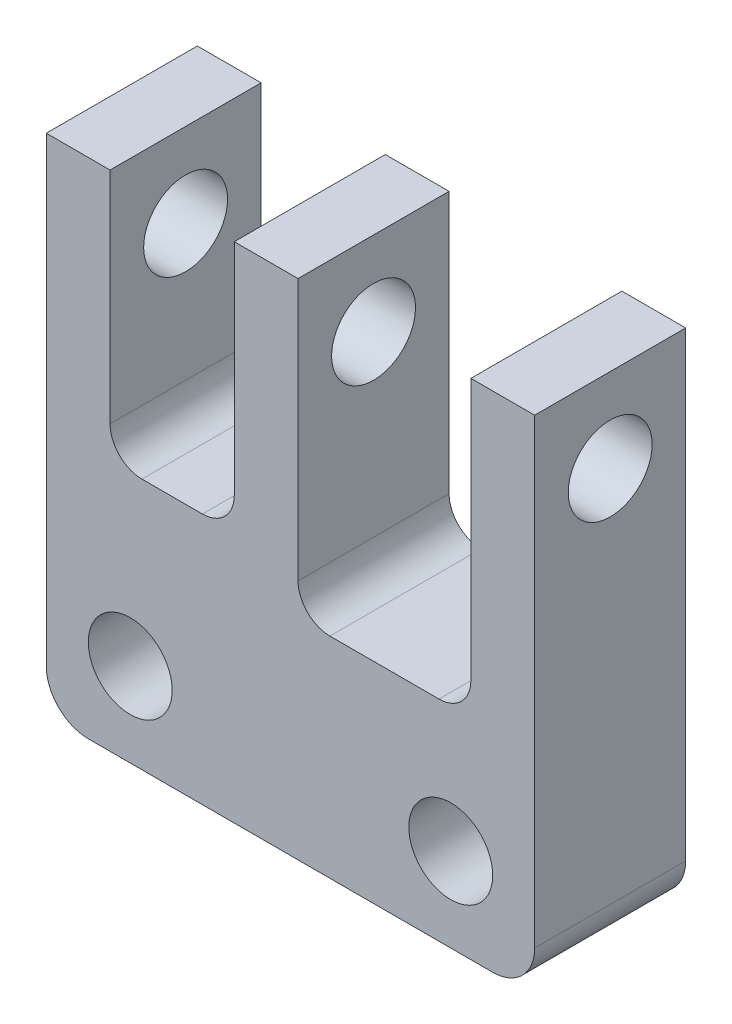
ISO-10303-21;
HEADER;
FILE_DESCRIPTION(('STEP AP214'),'2;1');
FILE_NAME('part.step','',(''),(''),'','','');
FILE_SCHEMA(('AUTOMOTIVE_DESIGN { 1 0 10303 214 1 1 1 1 }'));
ENDSEC;
DATA;
#1=APPLICATION_CONTEXT('core data for automotive mechanical design processes');
#2=APPLICATION_PROTOCOL_DEFINITION('international standard','automotive_design',2000,#1);
#3=PRODUCT_CONTEXT('',#1,'mechanical');
#4=PRODUCT('Part','Part','',(#3));
#5=PRODUCT_RELATED_PRODUCT_CATEGORY('part','',(#4));
#6=PRODUCT_DEFINITION_FORMATION('','',#4);
#7=PRODUCT_DEFINITION_CONTEXT('part definition',#1,'design');
#8=PRODUCT_DEFINITION('design','',#6,#7);
#9=PRODUCT_DEFINITION_SHAPE('','',#8);
#10=(LENGTH_UNIT() NAMED_UNIT(*) SI_UNIT(.MILLI.,.METRE.));
#11=(NAMED_UNIT(*) PLANE_ANGLE_UNIT() SI_UNIT($,.RADIAN.));
#12=(NAMED_UNIT(*) SI_UNIT($,.STERADIAN.) SOLID_ANGLE_UNIT());
#13=UNCERTAINTY_MEASURE_WITH_UNIT(LENGTH_MEASURE(1.E-05),#10,'distance_accuracy_value','');
#14=(GEOMETRIC_REPRESENTATION_CONTEXT(3) GLOBAL_UNCERTAINTY_ASSIGNED_CONTEXT((#13)) GLOBAL_UNIT_ASSIGNED_CONTEXT((#10,
#11,#12)) REPRESENTATION_CONTEXT('',''));
#15=CARTESIAN_POINT('',(0.,0.,0.));
#16=DIRECTION('',(0.,0.,1.));
#17=DIRECTION('',(1.,0.,0.));
#18=AXIS2_PLACEMENT_3D('',#15,#16,#17);
#19=CARTESIAN_POINT('',(0.,3.,0.));
#20=DIRECTION('',(0.,-1.,0.));
#21=DIRECTION('',(0.,0.,-1.));
#22=AXIS2_PLACEMENT_3D('',#19,#20,#21);
#23=PLANE('',#22);
#24=DIRECTION('',(-1.,0.,0.));
#25=VECTOR('',#24,1.);
#26=CARTESIAN_POINT('',(-1.455,3.,-0.45));
#27=LINE('',#26,#25);
#28=CARTESIAN_POINT('',(0.0450000000000003,3.,-0.45));
#29=VERTEX_POINT('',#28);
#30=CARTESIAN_POINT('',(-0.335,3.,-0.45));
#31=VERTEX_POINT('',#30);
#32=EDGE_CURVE('E209',#29,#31,#27,.T.);
#33=ORIENTED_EDGE('',*,*,#32,.T.);
#34=DIRECTION('',(0.,0.,1.));
#35=VECTOR('',#34,1.);
#36=CARTESIAN_POINT('',(-0.335,3.,0.));
#37=LINE('',#36,#35);
#38=CARTESIAN_POINT('',(-0.335,3.,0.45));
#39=VERTEX_POINT('',#38);
#40=EDGE_CURVE('E11',#31,#39,#37,.T.);
#41=ORIENTED_EDGE('',*,*,#40,.T.);
#42=DIRECTION('',(1.,0.,0.));
#43=VECTOR('',#42,1.);
#44=CARTESIAN_POINT('',(-1.455,3.,0.45));
#45=LINE('',#44,#43);
#46=CARTESIAN_POINT('',(0.0450000000000003,3.,0.45));
#47=VERTEX_POINT('',#46);
#48=EDGE_CURVE('E193',#39,#47,#45,.T.);
#49=ORIENTED_EDGE('',*,*,#48,.T.);
#50=DIRECTION('',(0.,0.,-1.));
#51=VECTOR('',#50,1.);
#52=CARTESIAN_POINT('',(0.0450000000000003,3.,0.));
#53=LINE('',#52,#51);
#54=EDGE_CURVE('E390',#47,#29,#53,.T.);
#55=ORIENTED_EDGE('',*,*,#54,.T.);
#56=EDGE_LOOP('',(#33,#41,#49,#55));
#57=FACE_BOUND('',#56,.T.);
#58=ADVANCED_FACE('F43',(#57),#23,.F.);
#59=CARTESIAN_POINT('',(1.455,3.,-0.45));
#60=VERTEX_POINT('',#59);
#61=CARTESIAN_POINT('',(1.075,3.,-0.45));
#62=VERTEX_POINT('',#61);
#63=EDGE_CURVE('E208',#60,#62,#27,.T.);
#64=ORIENTED_EDGE('',*,*,#63,.T.);
#65=DIRECTION('',(0.,0.,1.));
#66=VECTOR('',#65,1.);
#67=CARTESIAN_POINT('',(1.075,3.,0.));
#68=LINE('',#67,#66);
#69=CARTESIAN_POINT('',(1.075,3.,0.45));
#70=VERTEX_POINT('',#69);
#71=EDGE_CURVE('E179',#62,#70,#68,.T.);
#72=ORIENTED_EDGE('',*,*,#71,.T.);
#73=CARTESIAN_POINT('',(1.455,3.,0.45));
#74=VERTEX_POINT('',#73);
#75=EDGE_CURVE('E198',#70,#74,#45,.T.);
#76=ORIENTED_EDGE('',*,*,#75,.T.);
#77=DIRECTION('',(0.,0.,-1.));
#78=VECTOR('',#77,1.);
#79=CARTESIAN_POINT('',(1.455,3.,0.45));
#80=LINE('',#79,#78);
#81=EDGE_CURVE('E212',#74,#60,#80,.T.);
#82=ORIENTED_EDGE('',*,*,#81,.T.);
#83=EDGE_LOOP('',(#64,#72,#76,#82));
#84=FACE_BOUND('',#83,.T.);
#85=ADVANCED_FACE('F335',(#84),#23,.F.);
#86=CARTESIAN_POINT('',(1.455,3.,0.45));
#87=DIRECTION('',(-1.,0.,0.));
#88=DIRECTION('',(0.,0.,1.));
#89=AXIS2_PLACEMENT_3D('',#86,#87,#88);
#90=PLANE('',#89);
#91=CARTESIAN_POINT('',(1.455,2.5,0.));
#92=DIRECTION('',(1.,0.,0.));
#93=DIRECTION('',(0.,0.,-1.));
#94=AXIS2_PLACEMENT_3D('',#91,#92,#93);
#95=CIRCLE('',#94,0.25);
#96=CARTESIAN_POINT('',(1.455,2.5,-0.25));
#97=VERTEX_POINT('',#96);
#98=EDGE_CURVE('E305',#97,#97,#95,.T.);
#99=ORIENTED_EDGE('',*,*,#98,.F.);
#100=EDGE_LOOP('',(#99));
#101=FACE_BOUND('',#100,.T.);
#102=DIRECTION('',(0.,-1.,0.));
#103=VECTOR('',#102,1.);
#104=CARTESIAN_POINT('',(1.455,3.,0.45));
#105=LINE('',#104,#103);
#106=CARTESIAN_POINT('',(1.455,0.25,0.45));
#107=VERTEX_POINT('',#106);
#108=EDGE_CURVE('E195',#74,#107,#105,.T.);
#109=ORIENTED_EDGE('',*,*,#108,.T.);
#110=DIRECTION('',(0.,0.,-1.));
#111=VECTOR('',#110,1.);
#112=CARTESIAN_POINT('',(1.455,0.25,-0.45));
#113=LINE('',#112,#111);
#114=CARTESIAN_POINT('',(1.455,0.25,-0.45));
#115=VERTEX_POINT('',#114);
#116=EDGE_CURVE('E381',#107,#115,#113,.T.);
#117=ORIENTED_EDGE('',*,*,#116,.T.);
#118=DIRECTION('',(0.,-1.,0.));
#119=VECTOR('',#118,1.);
#120=CARTESIAN_POINT('',(1.455,3.,-0.45));
#121=LINE('',#120,#119);
#122=EDGE_CURVE('E397',#60,#115,#121,.T.);
#123=ORIENTED_EDGE('',*,*,#122,.F.);
#124=ORIENTED_EDGE('',*,*,#81,.F.);
#125=EDGE_LOOP('',(#109,#117,#123,#124));
#126=FACE_BOUND('',#125,.T.);
#127=ADVANCED_FACE('F338',(#101,#126),#90,.F.);
#128=CARTESIAN_POINT('',(-1.455,3.,-0.45));
#129=DIRECTION('',(0.,0.,1.));
#130=DIRECTION('',(1.,0.,0.));
#131=AXIS2_PLACEMENT_3D('',#128,#129,#130);
#132=PLANE('',#131);
#133=CARTESIAN_POINT('',(-0.955,0.5,-0.45));
#134=DIRECTION('',(0.,0.,1.));
#135=DIRECTION('',(1.,0.,0.));
#136=AXIS2_PLACEMENT_3D('',#133,#134,#135);
#137=CIRCLE('',#136,0.25);
#138=CARTESIAN_POINT('',(-0.705,0.5,-0.45));
#139=VERTEX_POINT('',#138);
#140=EDGE_CURVE('E266',#139,#139,#137,.T.);
#141=ORIENTED_EDGE('',*,*,#140,.T.);
#142=EDGE_LOOP('',(#141));
#143=FACE_BOUND('',#142,.T.);
#144=CARTESIAN_POINT('',(0.955,0.5,-0.45));
#145=DIRECTION('',(0.,0.,1.));
#146=DIRECTION('',(1.,0.,0.));
#147=AXIS2_PLACEMENT_3D('',#144,#145,#146);
#148=CIRCLE('',#147,0.25);
#149=CARTESIAN_POINT('',(1.205,0.5,-0.45));
#150=VERTEX_POINT('',#149);
#151=EDGE_CURVE('E285',#150,#150,#148,.T.);
#152=ORIENTED_EDGE('',*,*,#151,.T.);
#153=EDGE_LOOP('',(#152));
#154=FACE_BOUND('',#153,.T.);
#155=CARTESIAN_POINT('',(-0.525,1.69,-0.45));
#156=DIRECTION('',(0.,0.,1.));
#157=DIRECTION('',(1.,0.,0.));
#158=AXIS2_PLACEMENT_3D('',#155,#156,#157);
#159=CIRCLE('',#158,0.19);
#160=CARTESIAN_POINT('',(-0.525000000000001,1.5,-0.45));
#161=VERTEX_POINT('',#160);
#162=CARTESIAN_POINT('',(-0.335,1.69,-0.45));
#163=VERTEX_POINT('',#162);
#164=EDGE_CURVE('E220',#161,#163,#159,.T.);
#165=ORIENTED_EDGE('',*,*,#164,.T.);
#166=DIRECTION('',(0.,1.,0.));
#167=VECTOR('',#166,1.);
#168=CARTESIAN_POINT('',(-0.335,3.,-0.45));
#169=LINE('',#168,#167);
#170=EDGE_CURVE('E237',#163,#31,#169,.T.);
#171=ORIENTED_EDGE('',*,*,#170,.T.);
#172=ORIENTED_EDGE('',*,*,#32,.F.);
#173=DIRECTION('',(0.,-1.,0.));
#174=VECTOR('',#173,1.);
#175=CARTESIAN_POINT('',(0.0450000000000003,3.,-0.45));
#176=LINE('',#175,#174);
#177=CARTESIAN_POINT('',(0.0450000000000003,1.44,-0.45));
#178=VERTEX_POINT('',#177);
#179=EDGE_CURVE('E66',#29,#178,#176,.T.);
#180=ORIENTED_EDGE('',*,*,#179,.T.);
#181=CARTESIAN_POINT('',(0.235,1.44,-0.45));
#182=DIRECTION('',(0.,0.,1.));
#183=DIRECTION('',(1.,0.,0.));
#184=AXIS2_PLACEMENT_3D('',#181,#182,#183);
#185=CIRCLE('',#184,0.19);
#186=CARTESIAN_POINT('',(0.235000000000002,1.25,-0.45));
#187=VERTEX_POINT('',#186);
#188=EDGE_CURVE('E235',#178,#187,#185,.T.);
#189=ORIENTED_EDGE('',*,*,#188,.T.);
#190=DIRECTION('',(1.,0.,0.));
#191=VECTOR('',#190,1.);
#192=CARTESIAN_POINT('',(-1.455,1.25,-0.45));
#193=LINE('',#192,#191);
#194=CARTESIAN_POINT('',(0.884999999999999,1.25,-0.45));
#195=VERTEX_POINT('',#194);
#196=EDGE_CURVE('E230',#187,#195,#193,.T.);
#197=ORIENTED_EDGE('',*,*,#196,.T.);
#198=CARTESIAN_POINT('',(0.885,1.44,-0.45));
#199=DIRECTION('',(0.,0.,1.));
#200=DIRECTION('',(1.,0.,0.));
#201=AXIS2_PLACEMENT_3D('',#198,#199,#200);
#202=CIRCLE('',#201,0.19);
#203=CARTESIAN_POINT('',(1.075,1.44,-0.45));
#204=VERTEX_POINT('',#203);
#205=EDGE_CURVE('E227',#195,#204,#202,.T.);
#206=ORIENTED_EDGE('',*,*,#205,.T.);
#207=DIRECTION('',(0.,1.,0.));
#208=VECTOR('',#207,1.);
#209=CARTESIAN_POINT('',(1.075,3.,-0.45));
#210=LINE('',#209,#208);
#211=EDGE_CURVE('E238',#204,#62,#210,.T.);
#212=ORIENTED_EDGE('',*,*,#211,.T.);
#213=ORIENTED_EDGE('',*,*,#63,.F.);
#214=ORIENTED_EDGE('',*,*,#122,.T.);
#215=CARTESIAN_POINT('',(1.205,0.25,-0.45));
#216=DIRECTION('',(0.,0.,1.));
#217=DIRECTION('',(1.,0.,0.));
#218=AXIS2_PLACEMENT_3D('',#215,#216,#217);
#219=CIRCLE('',#218,0.25);
#220=CARTESIAN_POINT('',(1.205,0.,-0.45));
#221=VERTEX_POINT('',#220);
#222=EDGE_CURVE('E414',#115,#221,#219,.F.);
#223=ORIENTED_EDGE('',*,*,#222,.T.);
#224=DIRECTION('',(-1.,0.,0.));
#225=VECTOR('',#224,1.);
#226=CARTESIAN_POINT('',(-1.455,0.,-0.45));
#227=LINE('',#226,#225);
#228=CARTESIAN_POINT('',(-1.205,0.,-0.45));
#229=VERTEX_POINT('',#228);
#230=EDGE_CURVE('E219',#221,#229,#227,.T.);
#231=ORIENTED_EDGE('',*,*,#230,.T.);
#232=CARTESIAN_POINT('',(-1.205,0.25,-0.45));
#233=DIRECTION('',(0.,0.,1.));
#234=DIRECTION('',(1.,0.,0.));
#235=AXIS2_PLACEMENT_3D('',#232,#233,#234);
#236=CIRCLE('',#235,0.25);
#237=CARTESIAN_POINT('',(-1.455,0.25,-0.45));
#238=VERTEX_POINT('',#237);
#239=EDGE_CURVE('E404',#229,#238,#236,.F.);
#240=ORIENTED_EDGE('',*,*,#239,.T.);
#241=DIRECTION('',(0.,-1.,0.));
#242=VECTOR('',#241,1.);
#243=CARTESIAN_POINT('',(-1.455,3.,-0.45));
#244=LINE('',#243,#242);
#245=CARTESIAN_POINT('',(-1.455,3.,-0.45));
#246=VERTEX_POINT('',#245);
#247=EDGE_CURVE('E405',#246,#238,#244,.T.);
#248=ORIENTED_EDGE('',*,*,#247,.F.);
#249=CARTESIAN_POINT('',(-1.075,3.,-0.45));
#250=VERTEX_POINT('',#249);
#251=EDGE_CURVE('E215',#250,#246,#27,.T.);
#252=ORIENTED_EDGE('',*,*,#251,.F.);
#253=DIRECTION('',(0.,-1.,0.));
#254=VECTOR('',#253,1.);
#255=CARTESIAN_POINT('',(-1.075,3.,-0.45));
#256=LINE('',#255,#254);
#257=CARTESIAN_POINT('',(-1.075,1.69,-0.45));
#258=VERTEX_POINT('',#257);
#259=EDGE_CURVE('E56',#250,#258,#256,.T.);
#260=ORIENTED_EDGE('',*,*,#259,.T.);
#261=CARTESIAN_POINT('',(-0.885,1.69,-0.45));
#262=DIRECTION('',(0.,0.,1.));
#263=DIRECTION('',(1.,0.,0.));
#264=AXIS2_PLACEMENT_3D('',#261,#262,#263);
#265=CIRCLE('',#264,0.19);
#266=CARTESIAN_POINT('',(-0.884999999999999,1.5,-0.45));
#267=VERTEX_POINT('',#266);
#268=EDGE_CURVE('E221',#258,#267,#265,.T.);
#269=ORIENTED_EDGE('',*,*,#268,.T.);
#270=DIRECTION('',(1.,0.,0.));
#271=VECTOR('',#270,1.);
#272=CARTESIAN_POINT('',(-1.455,1.5,-0.45));
#273=LINE('',#272,#271);
#274=EDGE_CURVE('E222',#267,#161,#273,.T.);
#275=ORIENTED_EDGE('',*,*,#274,.T.);
#276=EDGE_LOOP('',(#165,#171,#172,#180,#189,#197,#206,#212,#213,#214,#223,#231,#240,#248,#252,
#260,#269,#275));
#277=FACE_BOUND('',#276,.T.);
#278=ADVANCED_FACE('F357',(#143,#154,#277),#132,.F.);
#279=CARTESIAN_POINT('',(-1.455,3.,0.45));
#280=DIRECTION('',(1.,0.,0.));
#281=DIRECTION('',(0.,0.,-1.));
#282=AXIS2_PLACEMENT_3D('',#279,#280,#281);
#283=PLANE('',#282);
#284=CARTESIAN_POINT('',(-1.455,2.5,0.));
#285=DIRECTION('',(1.,0.,0.));
#286=DIRECTION('',(0.,0.,-1.));
#287=AXIS2_PLACEMENT_3D('',#284,#285,#286);
#288=CIRCLE('',#287,0.25);
#289=CARTESIAN_POINT('',(-1.455,2.5,-0.25));
#290=VERTEX_POINT('',#289);
#291=EDGE_CURVE('E308',#290,#290,#288,.T.);
#292=ORIENTED_EDGE('',*,*,#291,.T.);
#293=EDGE_LOOP('',(#292));
#294=FACE_BOUND('',#293,.T.);
#295=ORIENTED_EDGE('',*,*,#247,.T.);
#296=DIRECTION('',(0.,0.,1.));
#297=VECTOR('',#296,1.);
#298=CARTESIAN_POINT('',(-1.455,0.25,0.45));
#299=LINE('',#298,#297);
#300=CARTESIAN_POINT('',(-1.455,0.25,0.45));
#301=VERTEX_POINT('',#300);
#302=EDGE_CURVE('E382',#238,#301,#299,.T.);
#303=ORIENTED_EDGE('',*,*,#302,.T.);
#304=DIRECTION('',(0.,-1.,0.));
#305=VECTOR('',#304,1.);
#306=CARTESIAN_POINT('',(-1.455,3.,0.45));
#307=LINE('',#306,#305);
#308=CARTESIAN_POINT('',(-1.455,3.,0.45));
#309=VERTEX_POINT('',#308);
#310=EDGE_CURVE('E196',#309,#301,#307,.T.);
#311=ORIENTED_EDGE('',*,*,#310,.F.);
#312=DIRECTION('',(0.,0.,1.));
#313=VECTOR('',#312,1.);
#314=CARTESIAN_POINT('',(-1.455,3.,0.45));
#315=LINE('',#314,#313);
#316=EDGE_CURVE('E194',#246,#309,#315,.T.);
#317=ORIENTED_EDGE('',*,*,#316,.F.);
#318=EDGE_LOOP('',(#295,#303,#311,#317));
#319=FACE_BOUND('',#318,.T.);
#320=ADVANCED_FACE('F352',(#294,#319),#283,.F.);
#321=CARTESIAN_POINT('',(-1.455,3.,0.45));
#322=DIRECTION('',(0.,0.,-1.));
#323=DIRECTION('',(-1.,0.,0.));
#324=AXIS2_PLACEMENT_3D('',#321,#322,#323);
#325=PLANE('',#324);
#326=CARTESIAN_POINT('',(-0.955,0.5,0.45));
#327=DIRECTION('',(0.,0.,1.));
#328=DIRECTION('',(1.,0.,0.));
#329=AXIS2_PLACEMENT_3D('',#326,#327,#328);
#330=CIRCLE('',#329,0.25);
#331=CARTESIAN_POINT('',(-0.705,0.5,0.45));
#332=VERTEX_POINT('',#331);
#333=EDGE_CURVE('E290',#332,#332,#330,.T.);
#334=ORIENTED_EDGE('',*,*,#333,.F.);
#335=EDGE_LOOP('',(#334));
#336=FACE_BOUND('',#335,.T.);
#337=CARTESIAN_POINT('',(0.955,0.5,0.45));
#338=DIRECTION('',(0.,0.,1.));
#339=DIRECTION('',(1.,0.,0.));
#340=AXIS2_PLACEMENT_3D('',#337,#338,#339);
#341=CIRCLE('',#340,0.25);
#342=CARTESIAN_POINT('',(1.205,0.5,0.45));
#343=VERTEX_POINT('',#342);
#344=EDGE_CURVE('E288',#343,#343,#341,.T.);
#345=ORIENTED_EDGE('',*,*,#344,.F.);
#346=EDGE_LOOP('',(#345));
#347=FACE_BOUND('',#346,.T.);
#348=ORIENTED_EDGE('',*,*,#48,.F.);
#349=DIRECTION('',(0.,1.,0.));
#350=VECTOR('',#349,1.);
#351=CARTESIAN_POINT('',(-0.335,1.69,0.45));
#352=LINE('',#351,#350);
#353=CARTESIAN_POINT('',(-0.335,1.69,0.45));
#354=VERTEX_POINT('',#353);
#355=EDGE_CURVE('E269',#354,#39,#352,.T.);
#356=ORIENTED_EDGE('',*,*,#355,.F.);
#357=CARTESIAN_POINT('',(-0.525,1.69,0.45));
#358=DIRECTION('',(0.,0.,1.));
#359=DIRECTION('',(1.,0.,0.));
#360=AXIS2_PLACEMENT_3D('',#357,#358,#359);
#361=CIRCLE('',#360,0.19);
#362=CARTESIAN_POINT('',(-0.525000000000001,1.5,0.45));
#363=VERTEX_POINT('',#362);
#364=EDGE_CURVE('E277',#363,#354,#361,.T.);
#365=ORIENTED_EDGE('',*,*,#364,.F.);
#366=DIRECTION('',(1.,0.,0.));
#367=VECTOR('',#366,1.);
#368=CARTESIAN_POINT('',(-0.884999999999999,1.5,0.45));
#369=LINE('',#368,#367);
#370=CARTESIAN_POINT('',(-0.884999999999999,1.5,0.45));
#371=VERTEX_POINT('',#370);
#372=EDGE_CURVE('E276',#371,#363,#369,.T.);
#373=ORIENTED_EDGE('',*,*,#372,.F.);
#374=CARTESIAN_POINT('',(-0.885,1.69,0.45));
#375=DIRECTION('',(0.,0.,1.));
#376=DIRECTION('',(1.,0.,0.));
#377=AXIS2_PLACEMENT_3D('',#374,#375,#376);
#378=CIRCLE('',#377,0.19);
#379=CARTESIAN_POINT('',(-1.075,1.69,0.45));
#380=VERTEX_POINT('',#379);
#381=EDGE_CURVE('E186',#380,#371,#378,.T.);
#382=ORIENTED_EDGE('',*,*,#381,.F.);
#383=DIRECTION('',(0.,-1.,0.));
#384=VECTOR('',#383,1.);
#385=CARTESIAN_POINT('',(-1.075,3.,0.45));
#386=LINE('',#385,#384);
#387=CARTESIAN_POINT('',(-1.075,3.,0.45));
#388=VERTEX_POINT('',#387);
#389=EDGE_CURVE('E171',#388,#380,#386,.T.);
#390=ORIENTED_EDGE('',*,*,#389,.F.);
#391=EDGE_CURVE('E181',#309,#388,#45,.T.);
#392=ORIENTED_EDGE('',*,*,#391,.F.);
#393=ORIENTED_EDGE('',*,*,#310,.T.);
#394=CARTESIAN_POINT('',(-1.205,0.25,0.45));
#395=DIRECTION('',(0.,0.,-1.));
#396=DIRECTION('',(-1.,0.,0.));
#397=AXIS2_PLACEMENT_3D('',#394,#395,#396);
#398=CIRCLE('',#397,0.25);
#399=CARTESIAN_POINT('',(-1.205,0.,0.45));
#400=VERTEX_POINT('',#399);
#401=EDGE_CURVE('E383',#301,#400,#398,.F.);
#402=ORIENTED_EDGE('',*,*,#401,.T.);
#403=DIRECTION('',(1.,0.,0.));
#404=VECTOR('',#403,1.);
#405=CARTESIAN_POINT('',(-1.455,0.,0.45));
#406=LINE('',#405,#404);
#407=CARTESIAN_POINT('',(1.205,0.,0.45));
#408=VERTEX_POINT('',#407);
#409=EDGE_CURVE('E216',#400,#408,#406,.T.);
#410=ORIENTED_EDGE('',*,*,#409,.T.);
#411=CARTESIAN_POINT('',(1.205,0.25,0.45));
#412=DIRECTION('',(0.,0.,-1.));
#413=DIRECTION('',(-1.,0.,0.));
#414=AXIS2_PLACEMENT_3D('',#411,#412,#413);
#415=CIRCLE('',#414,0.25);
#416=EDGE_CURVE('E378',#408,#107,#415,.F.);
#417=ORIENTED_EDGE('',*,*,#416,.T.);
#418=ORIENTED_EDGE('',*,*,#108,.F.);
#419=ORIENTED_EDGE('',*,*,#75,.F.);
#420=DIRECTION('',(0.,1.,0.));
#421=VECTOR('',#420,1.);
#422=CARTESIAN_POINT('',(1.075,3.,0.45));
#423=LINE('',#422,#421);
#424=CARTESIAN_POINT('',(1.075,1.44,0.45));
#425=VERTEX_POINT('',#424);
#426=EDGE_CURVE('E250',#425,#70,#423,.T.);
#427=ORIENTED_EDGE('',*,*,#426,.F.);
#428=CARTESIAN_POINT('',(0.885,1.44,0.45));
#429=DIRECTION('',(0.,0.,1.));
#430=DIRECTION('',(-1.,0.,0.));
#431=AXIS2_PLACEMENT_3D('',#428,#429,#430);
#432=CIRCLE('',#431,0.19);
#433=CARTESIAN_POINT('',(0.884999999999999,1.25,0.45));
#434=VERTEX_POINT('',#433);
#435=EDGE_CURVE('E255',#434,#425,#432,.T.);
#436=ORIENTED_EDGE('',*,*,#435,.F.);
#437=DIRECTION('',(1.,0.,0.));
#438=VECTOR('',#437,1.);
#439=CARTESIAN_POINT('',(0.884999999999999,1.25,0.45));
#440=LINE('',#439,#438);
#441=CARTESIAN_POINT('',(0.235000000000002,1.25,0.45));
#442=VERTEX_POINT('',#441);
#443=EDGE_CURVE('E260',#442,#434,#440,.T.);
#444=ORIENTED_EDGE('',*,*,#443,.F.);
#445=CARTESIAN_POINT('',(0.235,1.44,0.45));
#446=DIRECTION('',(0.,0.,1.));
#447=DIRECTION('',(-1.,0.,0.));
#448=AXIS2_PLACEMENT_3D('',#445,#446,#447);
#449=CIRCLE('',#448,0.19);
#450=CARTESIAN_POINT('',(0.0450000000000003,1.44,0.45));
#451=VERTEX_POINT('',#450);
#452=EDGE_CURVE('E257',#451,#442,#449,.T.);
#453=ORIENTED_EDGE('',*,*,#452,.F.);
#454=DIRECTION('',(0.,-1.,0.));
#455=VECTOR('',#454,1.);
#456=CARTESIAN_POINT('',(0.0450000000000003,1.44,0.45));
#457=LINE('',#456,#455);
#458=EDGE_CURVE('E263',#47,#451,#457,.T.);
#459=ORIENTED_EDGE('',*,*,#458,.F.);
#460=EDGE_LOOP('',(#348,#356,#365,#373,#382,#390,#392,#393,#402,#410,#417,#418,#419,#427,#436,
#444,#453,#459));
#461=FACE_BOUND('',#460,.T.);
#462=ADVANCED_FACE('F182',(#336,#347,#461),#325,.F.);
#463=ORIENTED_EDGE('',*,*,#391,.T.);
#464=DIRECTION('',(0.,0.,-1.));
#465=VECTOR('',#464,1.);
#466=CARTESIAN_POINT('',(-1.075,3.,0.));
#467=LINE('',#466,#465);
#468=EDGE_CURVE('E55',#388,#250,#467,.T.);
#469=ORIENTED_EDGE('',*,*,#468,.T.);
#470=ORIENTED_EDGE('',*,*,#251,.T.);
#471=ORIENTED_EDGE('',*,*,#316,.T.);
#472=EDGE_LOOP('',(#463,#469,#470,#471));
#473=FACE_BOUND('',#472,.T.);
#474=ADVANCED_FACE('F188',(#473),#23,.F.);
#475=CARTESIAN_POINT('',(0.,0.,0.));
#476=DIRECTION('',(0.,-1.,0.));
#477=DIRECTION('',(0.,0.,-1.));
#478=AXIS2_PLACEMENT_3D('',#475,#476,#477);
#479=PLANE('',#478);
#480=ORIENTED_EDGE('',*,*,#230,.F.);
#481=DIRECTION('',(0.,0.,-1.));
#482=VECTOR('',#481,1.);
#483=CARTESIAN_POINT('',(1.205,0.,0.45));
#484=LINE('',#483,#482);
#485=EDGE_CURVE('E377',#221,#408,#484,.F.);
#486=ORIENTED_EDGE('',*,*,#485,.T.);
#487=ORIENTED_EDGE('',*,*,#409,.F.);
#488=DIRECTION('',(0.,0.,1.));
#489=VECTOR('',#488,1.);
#490=CARTESIAN_POINT('',(-1.205,0.,-0.45));
#491=LINE('',#490,#489);
#492=EDGE_CURVE('E415',#400,#229,#491,.F.);
#493=ORIENTED_EDGE('',*,*,#492,.T.);
#494=EDGE_LOOP('',(#480,#486,#487,#493));
#495=FACE_BOUND('',#494,.T.);
#496=ADVANCED_FACE('F343',(#495),#479,.T.);
#497=CARTESIAN_POINT('',(1.205,0.25,0.45));
#498=DIRECTION('',(0.,0.,1.));
#499=DIRECTION('',(1.,0.,0.));
#500=AXIS2_PLACEMENT_3D('',#497,#498,#499);
#501=CYLINDRICAL_SURFACE('',#500,0.25);
#502=ORIENTED_EDGE('',*,*,#416,.F.);
#503=ORIENTED_EDGE('',*,*,#485,.F.);
#504=ORIENTED_EDGE('',*,*,#222,.F.);
#505=ORIENTED_EDGE('',*,*,#116,.F.);
#506=EDGE_LOOP('',(#502,#503,#504,#505));
#507=FACE_BOUND('',#506,.T.);
#508=ADVANCED_FACE('F349',(#507),#501,.T.);
#509=CARTESIAN_POINT('',(-1.205,0.25,0.45));
#510=DIRECTION('',(0.,0.,-1.));
#511=DIRECTION('',(-1.,0.,0.));
#512=AXIS2_PLACEMENT_3D('',#509,#510,#511);
#513=CYLINDRICAL_SURFACE('',#512,0.25);
#514=ORIENTED_EDGE('',*,*,#239,.F.);
#515=ORIENTED_EDGE('',*,*,#492,.F.);
#516=ORIENTED_EDGE('',*,*,#401,.F.);
#517=ORIENTED_EDGE('',*,*,#302,.F.);
#518=EDGE_LOOP('',(#514,#515,#516,#517));
#519=FACE_BOUND('',#518,.T.);
#520=ADVANCED_FACE('F44',(#519),#513,.T.);
#521=CARTESIAN_POINT('',(0.885,1.44,-2.55));
#522=DIRECTION('',(0.,0.,1.));
#523=DIRECTION('',(1.,0.,0.));
#524=AXIS2_PLACEMENT_3D('',#521,#522,#523);
#525=CYLINDRICAL_SURFACE('',#524,0.19);
#526=DIRECTION('',(0.,0.,1.));
#527=VECTOR('',#526,1.);
#528=CARTESIAN_POINT('',(0.884999999999999,1.25,-2.55));
#529=LINE('',#528,#527);
#530=EDGE_CURVE('E247',#195,#434,#529,.T.);
#531=ORIENTED_EDGE('',*,*,#530,.T.);
#532=ORIENTED_EDGE('',*,*,#435,.T.);
#533=DIRECTION('',(0.,0.,1.));
#534=VECTOR('',#533,1.);
#535=CARTESIAN_POINT('',(1.075,1.44,-2.55));
#536=LINE('',#535,#534);
#537=EDGE_CURVE('E187',#204,#425,#536,.T.);
#538=ORIENTED_EDGE('',*,*,#537,.F.);
#539=ORIENTED_EDGE('',*,*,#205,.F.);
#540=EDGE_LOOP('',(#531,#532,#538,#539));
#541=FACE_BOUND('',#540,.T.);
#542=ADVANCED_FACE('F373',(#541),#525,.F.);
#543=CARTESIAN_POINT('',(0.884999999999999,1.25,-2.55));
#544=DIRECTION('',(0.,-1.,0.));
#545=DIRECTION('',(1.,0.,0.));
#546=AXIS2_PLACEMENT_3D('',#543,#544,#545);
#547=PLANE('',#546);
#548=DIRECTION('',(0.,0.,1.));
#549=VECTOR('',#548,1.);
#550=CARTESIAN_POINT('',(0.235000000000002,1.25,-2.55));
#551=LINE('',#550,#549);
#552=EDGE_CURVE('E246',#187,#442,#551,.T.);
#553=ORIENTED_EDGE('',*,*,#552,.T.);
#554=ORIENTED_EDGE('',*,*,#443,.T.);
#555=ORIENTED_EDGE('',*,*,#530,.F.);
#556=ORIENTED_EDGE('',*,*,#196,.F.);
#557=EDGE_LOOP('',(#553,#554,#555,#556));
#558=FACE_BOUND('',#557,.T.);
#559=ADVANCED_FACE('F442',(#558),#547,.F.);
#560=CARTESIAN_POINT('',(0.235,1.44,-2.55));
#561=DIRECTION('',(0.,0.,1.));
#562=DIRECTION('',(1.,0.,0.));
#563=AXIS2_PLACEMENT_3D('',#560,#561,#562);
#564=CYLINDRICAL_SURFACE('',#563,0.19);
#565=DIRECTION('',(0.,0.,1.));
#566=VECTOR('',#565,1.);
#567=CARTESIAN_POINT('',(0.0450000000000003,1.44,-2.55));
#568=LINE('',#567,#566);
#569=EDGE_CURVE('E245',#178,#451,#568,.T.);
#570=ORIENTED_EDGE('',*,*,#569,.T.);
#571=ORIENTED_EDGE('',*,*,#452,.T.);
#572=ORIENTED_EDGE('',*,*,#552,.F.);
#573=ORIENTED_EDGE('',*,*,#188,.F.);
#574=EDGE_LOOP('',(#570,#571,#572,#573));
#575=FACE_BOUND('',#574,.T.);
#576=ADVANCED_FACE('F440',(#575),#564,.F.);
#577=CARTESIAN_POINT('',(1.075,3.,-2.55));
#578=DIRECTION('',(1.,0.,0.));
#579=DIRECTION('',(0.,1.,0.));
#580=AXIS2_PLACEMENT_3D('',#577,#578,#579);
#581=PLANE('',#580);
#582=CARTESIAN_POINT('',(1.075,2.5,0.));
#583=DIRECTION('',(1.,0.,0.));
#584=DIRECTION('',(0.,1.,0.));
#585=AXIS2_PLACEMENT_3D('',#582,#583,#584);
#586=CIRCLE('',#585,0.25);
#587=CARTESIAN_POINT('',(1.075,2.75,0.));
#588=VERTEX_POINT('',#587);
#589=EDGE_CURVE('E295',#588,#588,#586,.T.);
#590=ORIENTED_EDGE('',*,*,#589,.T.);
#591=EDGE_LOOP('',(#590));
#592=FACE_BOUND('',#591,.T.);
#593=ORIENTED_EDGE('',*,*,#537,.T.);
#594=ORIENTED_EDGE('',*,*,#426,.T.);
#595=ORIENTED_EDGE('',*,*,#71,.F.);
#596=ORIENTED_EDGE('',*,*,#211,.F.);
#597=EDGE_LOOP('',(#593,#594,#595,#596));
#598=FACE_BOUND('',#597,.T.);
#599=ADVANCED_FACE('F441',(#592,#598),#581,.F.);
#600=CARTESIAN_POINT('',(0.0450000000000003,1.44,-2.55));
#601=DIRECTION('',(-1.,0.,0.));
#602=DIRECTION('',(0.,0.,1.));
#603=AXIS2_PLACEMENT_3D('',#600,#601,#602);
#604=PLANE('',#603);
#605=CARTESIAN_POINT('',(0.0450000000000003,2.5,0.));
#606=DIRECTION('',(-1.,0.,0.));
#607=DIRECTION('',(0.,0.,1.));
#608=AXIS2_PLACEMENT_3D('',#605,#606,#607);
#609=CIRCLE('',#608,0.25);
#610=CARTESIAN_POINT('',(0.0450000000000003,2.5,0.25));
#611=VERTEX_POINT('',#610);
#612=EDGE_CURVE('E297',#611,#611,#609,.T.);
#613=ORIENTED_EDGE('',*,*,#612,.T.);
#614=EDGE_LOOP('',(#613));
#615=FACE_BOUND('',#614,.T.);
#616=ORIENTED_EDGE('',*,*,#54,.F.);
#617=ORIENTED_EDGE('',*,*,#458,.T.);
#618=ORIENTED_EDGE('',*,*,#569,.F.);
#619=ORIENTED_EDGE('',*,*,#179,.F.);
#620=EDGE_LOOP('',(#616,#617,#618,#619));
#621=FACE_BOUND('',#620,.T.);
#622=ADVANCED_FACE('F434',(#615,#621),#604,.F.);
#623=CARTESIAN_POINT('',(-0.525,1.69,-2.55));
#624=DIRECTION('',(0.,0.,1.));
#625=DIRECTION('',(1.,0.,0.));
#626=AXIS2_PLACEMENT_3D('',#623,#624,#625);
#627=CYLINDRICAL_SURFACE('',#626,0.19);
#628=DIRECTION('',(0.,0.,1.));
#629=VECTOR('',#628,1.);
#630=CARTESIAN_POINT('',(-0.525000000000001,1.5,-2.55));
#631=LINE('',#630,#629);
#632=EDGE_CURVE('E275',#161,#363,#631,.T.);
#633=ORIENTED_EDGE('',*,*,#632,.T.);
#634=ORIENTED_EDGE('',*,*,#364,.T.);
#635=DIRECTION('',(0.,0.,1.));
#636=VECTOR('',#635,1.);
#637=CARTESIAN_POINT('',(-0.335,1.69,-2.55));
#638=LINE('',#637,#636);
#639=EDGE_CURVE('E243',#163,#354,#638,.T.);
#640=ORIENTED_EDGE('',*,*,#639,.F.);
#641=ORIENTED_EDGE('',*,*,#164,.F.);
#642=EDGE_LOOP('',(#633,#634,#640,#641));
#643=FACE_BOUND('',#642,.T.);
#644=ADVANCED_FACE('F428',(#643),#627,.F.);
#645=CARTESIAN_POINT('',(-0.884999999999999,1.5,-2.55));
#646=DIRECTION('',(0.,-1.,0.));
#647=DIRECTION('',(0.,0.,-1.));
#648=AXIS2_PLACEMENT_3D('',#645,#646,#647);
#649=PLANE('',#648);
#650=DIRECTION('',(0.,0.,1.));
#651=VECTOR('',#650,1.);
#652=CARTESIAN_POINT('',(-0.884999999999999,1.5,-2.55));
#653=LINE('',#652,#651);
#654=EDGE_CURVE('E267',#267,#371,#653,.T.);
#655=ORIENTED_EDGE('',*,*,#654,.T.);
#656=ORIENTED_EDGE('',*,*,#372,.T.);
#657=ORIENTED_EDGE('',*,*,#632,.F.);
#658=ORIENTED_EDGE('',*,*,#274,.F.);
#659=EDGE_LOOP('',(#655,#656,#657,#658));
#660=FACE_BOUND('',#659,.T.);
#661=ADVANCED_FACE('F474',(#660),#649,.F.);
#662=CARTESIAN_POINT('',(-0.885,1.69,-2.55));
#663=DIRECTION('',(0.,0.,1.));
#664=DIRECTION('',(1.,0.,0.));
#665=AXIS2_PLACEMENT_3D('',#662,#663,#664);
#666=CYLINDRICAL_SURFACE('',#665,0.19);
#667=DIRECTION('',(0.,0.,1.));
#668=VECTOR('',#667,1.);
#669=CARTESIAN_POINT('',(-1.075,1.69,-2.55));
#670=LINE('',#669,#668);
#671=EDGE_CURVE('E270',#258,#380,#670,.T.);
#672=ORIENTED_EDGE('',*,*,#671,.T.);
#673=ORIENTED_EDGE('',*,*,#381,.T.);
#674=ORIENTED_EDGE('',*,*,#654,.F.);
#675=ORIENTED_EDGE('',*,*,#268,.F.);
#676=EDGE_LOOP('',(#672,#673,#674,#675));
#677=FACE_BOUND('',#676,.T.);
#678=ADVANCED_FACE('F482',(#677),#666,.F.);
#679=CARTESIAN_POINT('',(-0.335,1.69,-2.55));
#680=DIRECTION('',(1.,0.,0.));
#681=DIRECTION('',(0.,1.,0.));
#682=AXIS2_PLACEMENT_3D('',#679,#680,#681);
#683=PLANE('',#682);
#684=CARTESIAN_POINT('',(-0.335,2.5,0.));
#685=DIRECTION('',(1.,0.,0.));
#686=DIRECTION('',(0.,1.,0.));
#687=AXIS2_PLACEMENT_3D('',#684,#685,#686);
#688=CIRCLE('',#687,0.25);
#689=CARTESIAN_POINT('',(-0.335,2.75,0.));
#690=VERTEX_POINT('',#689);
#691=EDGE_CURVE('E300',#690,#690,#688,.T.);
#692=ORIENTED_EDGE('',*,*,#691,.T.);
#693=EDGE_LOOP('',(#692));
#694=FACE_BOUND('',#693,.T.);
#695=ORIENTED_EDGE('',*,*,#639,.T.);
#696=ORIENTED_EDGE('',*,*,#355,.T.);
#697=ORIENTED_EDGE('',*,*,#40,.F.);
#698=ORIENTED_EDGE('',*,*,#170,.F.);
#699=EDGE_LOOP('',(#695,#696,#697,#698));
#700=FACE_BOUND('',#699,.T.);
#701=ADVANCED_FACE('F426',(#694,#700),#683,.F.);
#702=CARTESIAN_POINT('',(-1.075,3.,-2.55));
#703=DIRECTION('',(-1.,0.,0.));
#704=DIRECTION('',(0.,0.,1.));
#705=AXIS2_PLACEMENT_3D('',#702,#703,#704);
#706=PLANE('',#705);
#707=CARTESIAN_POINT('',(-1.075,2.5,0.));
#708=DIRECTION('',(-1.,0.,0.));
#709=DIRECTION('',(0.,0.,1.));
#710=AXIS2_PLACEMENT_3D('',#707,#708,#709);
#711=CIRCLE('',#710,0.25);
#712=CARTESIAN_POINT('',(-1.075,2.5,0.25));
#713=VERTEX_POINT('',#712);
#714=EDGE_CURVE('E50',#713,#713,#711,.T.);
#715=ORIENTED_EDGE('',*,*,#714,.T.);
#716=EDGE_LOOP('',(#715));
#717=FACE_BOUND('',#716,.T.);
#718=ORIENTED_EDGE('',*,*,#468,.F.);
#719=ORIENTED_EDGE('',*,*,#389,.T.);
#720=ORIENTED_EDGE('',*,*,#671,.F.);
#721=ORIENTED_EDGE('',*,*,#259,.F.);
#722=EDGE_LOOP('',(#718,#719,#720,#721));
#723=FACE_BOUND('',#722,.T.);
#724=ADVANCED_FACE('F168',(#717,#723),#706,.F.);
#725=CARTESIAN_POINT('',(0.955,0.5,-2.55));
#726=DIRECTION('',(0.,0.,1.));
#727=DIRECTION('',(1.,0.,0.));
#728=AXIS2_PLACEMENT_3D('',#725,#726,#727);
#729=CYLINDRICAL_SURFACE('',#728,0.25);
#730=ORIENTED_EDGE('',*,*,#344,.T.);
#731=EDGE_LOOP('',(#730));
#732=FACE_BOUND('',#731,.T.);
#733=ORIENTED_EDGE('',*,*,#151,.F.);
#734=EDGE_LOOP('',(#733));
#735=FACE_BOUND('',#734,.T.);
#736=ADVANCED_FACE('F326',(#732,#735),#729,.F.);
#737=CARTESIAN_POINT('',(-0.955,0.5,-2.55));
#738=DIRECTION('',(0.,0.,1.));
#739=DIRECTION('',(1.,0.,0.));
#740=AXIS2_PLACEMENT_3D('',#737,#738,#739);
#741=CYLINDRICAL_SURFACE('',#740,0.25);
#742=ORIENTED_EDGE('',*,*,#333,.T.);
#743=EDGE_LOOP('',(#742));
#744=FACE_BOUND('',#743,.T.);
#745=ORIENTED_EDGE('',*,*,#140,.F.);
#746=EDGE_LOOP('',(#745));
#747=FACE_BOUND('',#746,.T.);
#748=ADVANCED_FACE('F320',(#744,#747),#741,.F.);
#749=CARTESIAN_POINT('',(-1.455,2.5,0.));
#750=DIRECTION('',(1.,0.,0.));
#751=DIRECTION('',(0.,0.,-1.));
#752=AXIS2_PLACEMENT_3D('',#749,#750,#751);
#753=CYLINDRICAL_SURFACE('',#752,0.25);
#754=ORIENTED_EDGE('',*,*,#291,.F.);
#755=EDGE_LOOP('',(#754));
#756=FACE_BOUND('',#755,.T.);
#757=ORIENTED_EDGE('',*,*,#714,.F.);
#758=EDGE_LOOP('',(#757));
#759=FACE_BOUND('',#758,.T.);
#760=ADVANCED_FACE('F314',(#756,#759),#753,.F.);
#761=ORIENTED_EDGE('',*,*,#691,.F.);
#762=EDGE_LOOP('',(#761));
#763=FACE_BOUND('',#762,.T.);
#764=ORIENTED_EDGE('',*,*,#612,.F.);
#765=EDGE_LOOP('',(#764));
#766=FACE_BOUND('',#765,.T.);
#767=ADVANCED_FACE('F316',(#763,#766),#753,.F.);
#768=ORIENTED_EDGE('',*,*,#98,.T.);
#769=EDGE_LOOP('',(#768));
#770=FACE_BOUND('',#769,.T.);
#771=ORIENTED_EDGE('',*,*,#589,.F.);
#772=EDGE_LOOP('',(#771));
#773=FACE_BOUND('',#772,.T.);
#774=ADVANCED_FACE('F319',(#770,#773),#753,.F.);
#775=CLOSED_SHELL('',(#58,#85,#127,#278,#320,#462,#474,#496,#508,#520,#542,#559,#576,#599,#622,
#644,#661,#678,#701,#724,#736,#748,#760,#767,#774));
#776=MANIFOLD_SOLID_BREP('B2',#775);
#777=ADVANCED_BREP_SHAPE_REPRESENTATION('',(#18,#776),#14);
#778=SHAPE_DEFINITION_REPRESENTATION(#9,#777);
ENDSEC;
END-ISO-10303-21;
